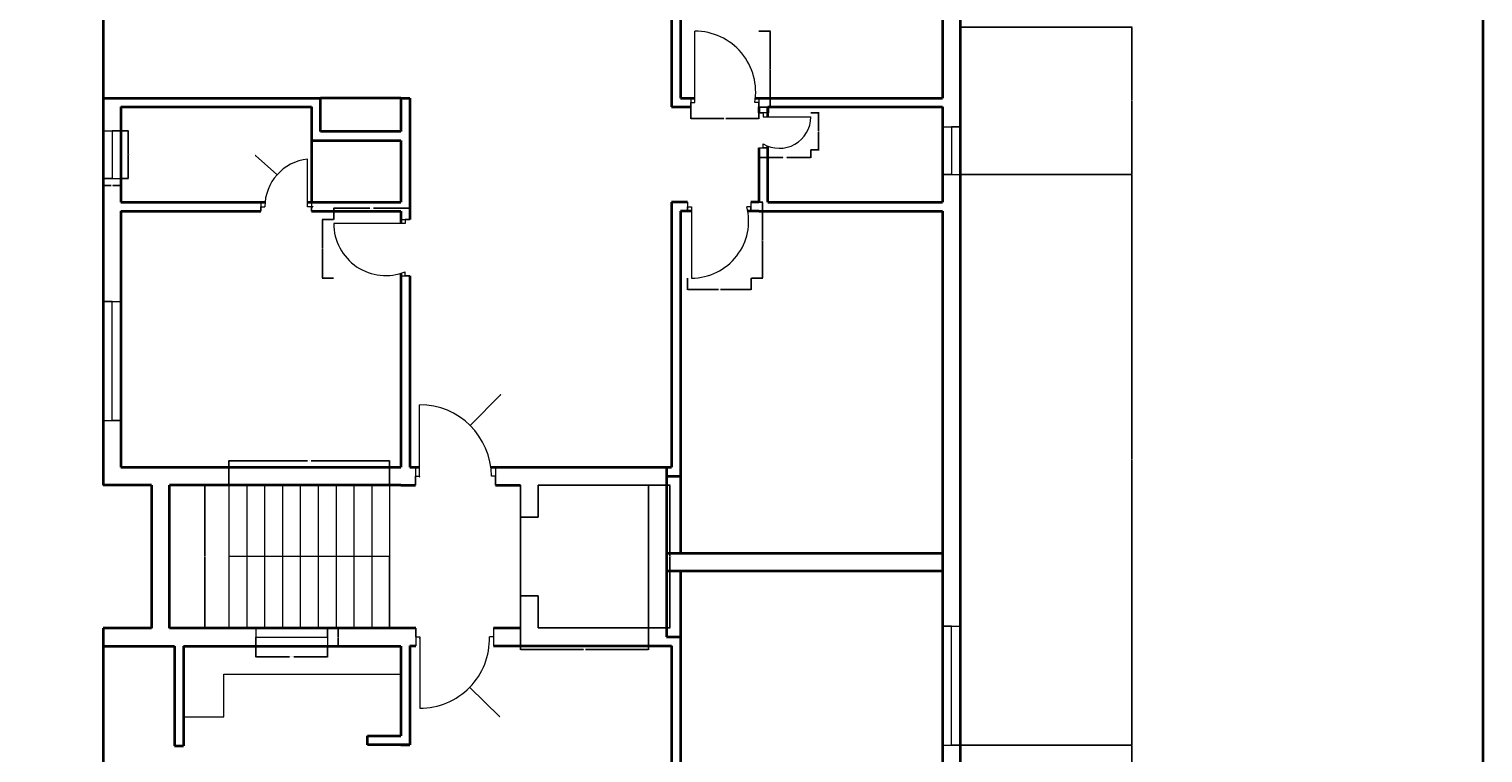
# Model space of a CAD drawing. Units: inches. Extents: x 2250 to 3547, y 1387 to 2604.
# Tile 5 of 11: x 2814 to 3547, y 1765 to 2129. Entities that reach past the tile are written whole.
import ezdxf

# ---------------------------------------------------------------- set-up
doc = ezdxf.new("R2010")
doc.units = ezdxf.units.IN
for name, color, linetype, lineweight in [('A-ANNO-DIMS', 2, 'Continuous', 18), ('A-ANNO-TTLB', 7, 'Continuous', 35), ('A-DOOR', 3, 'Continuous', 18), ('A-FLOR-CASE', 9, 'Continuous', 18), ('A-FLOR-EVTR', 6, 'Continuous', 25), ('A-FLOR-STRS', 7, 'Continuous', 18), ('A-GLAZ', 4, 'Continuous', 18), ('A-WALL', 7, 'Continuous', 35)]:
    doc.layers.add(name, color=color, linetype=linetype, lineweight=lineweight)
doc.styles.get("Standard").update_dxf_attribs({"font": 'arial.ttf'})
doc.dimstyles.get("Standard").update_dxf_attribs({"dimtxt": 0.18, "dimasz": 0.18, "dimexe": 0.18, "dimexo": 0.0625, "dimgap": 0.09, "dimtad": 0, "dimtih": 1, "dimtoh": 1, "dimdec": 4, "dimzin": 0, "dimdsep": 46, "dimtxsty": 'Standard', "dimcen": 0.09, "dimadec": 0, "dimazin": 0, "dimtfac": 1, "dimtdec": 4, "dimtofl": 0, "dimtmove": 0, "dimatfit": 3, "dimfxl": 1, "dimtolj": 1, "dimtzin": 0, "dimarcsym": 0})

# ---------------------------------------------------------------- blocks, each defined once
blk = doc.blocks.new('WIN-24')
for p, q in [((0, 24), (9, 24)), ((9, 24), (4.5, 24)), ((4.5, 24), (4.5, 0)), ((4.5, 0), (0, 0)), ((0, 0), (9, 0))]:
    blk.add_line(p, q)
blk = doc.blocks.new('WIN-60')
for p, q in [((0, 9), (0, 0)), ((60, 4.5), (60, 9)), ((60, 9), (60, 0)), ((0, 0), (0, 4.5)), ((0, 4.5), (60, 4.5))]:
    blk.add_line(p, q)
blk = doc.blocks.new('WIN-36')
for p, q in [((0, 9), (0, 0)), ((36, 4.5), (36, 9)), ((36, 9), (36, 0)), ((0, 0), (0, 4.5)), ((0, 4.5), (36, 4.5))]:
    blk.add_line(p, q)
blk = doc.blocks.new('DOOR-BED-NORTHEAST')
for p, q in [((2, 2.25), (2, 38.25)), ((0, 4.5), (0, 0)), ((0, 0), (0, 2.25)), ((0, 2.25), (2, 2.25)), ((34.25, 2.25), (32.25, 2.25)), ((34.25, 4.5), (34.25, 0)), ((34.25, 0), (34.25, 2.25))]:
    blk.add_line(p, q)
blk.add_arc((2, 7.54), 30.71, 350.07545, 90)
blk = doc.blocks.new('DOOR-BED-WEST-N')
for p, q in [((36, 26.33), (0, 26.33)), ((33.75, 28.33), (38.25, 28.33)), ((38.25, 28.33), (36, 28.33)), ((36, 28.33), (36, 26.33)), ((33.75, 0), (38.25, 0)), ((36, 0), (36, 2)), ((38.25, 0), (36, 0))]:
    blk.add_line(p, q)
blk.add_arc((26.22, 26.33), 26.22, 180, 291.89526)
blk = doc.blocks.new('DOOR-BATH-WEST-N')
for p, q in [((23.5, 2.25), (23.5, 26.25)), ((0, 4.5), (0, 0)), ((0, 0), (0, 2.25)), ((0, 2.25), (2, 2.25)), ((25.5, 2.25), (23.5, 2.25)), ((25.5, 4.5), (25.5, 0)), ((25.5, 0), (25.5, 2.25))]:
    blk.add_line(p, q)
blk.add_arc((26.15, 2.25), 24.15, 96.28991, 180)
blk = doc.blocks.new('DOOR-BATH-EAST-N')
for p, q in [((4.5, 17.63), (0, 17.63)), ((0, 17.63), (2.25, 17.63)), ((2.25, 17.63), (2.25, 15.63)), ((2.25, 15.63), (26.25, 15.63)), ((0, 0), (4.5, 0)), ((2.25, 0), (2.25, 2)), ((4.5, 0), (2.25, 0))]:
    blk.add_line(p, q)
blk.add_arc((10.38, 15.63), 15.87, 239.20063, 0)
blk = doc.blocks.new('DOOR-BED-EAST-N')
for p, q in [((0, 38.25), (0, 33.75)), ((31.84, 38.25), (31.84, 33.75)), ((0, 33.75), (0, 36)), ((0, 36), (2, 36)), ((2, 36), (2, 0)), ((31.84, 36), (29.84, 36)), ((31.84, 33.75), (31.84, 36))]:
    blk.add_line(p, q)
blk.add_arc((2, 28.77), 28.77, 270, 14.56312)
blk = doc.blocks.new('DOOR-LOBBY-NORTH')
for p, q in [((2, 4.5), (2, 40.5)), ((0, 9), (0, 0)), ((40.31, 9), (40.31, 0)), ((0, 0), (0, 4.5)), ((0, 4.5), (2, 4.5)), ((40.31, 4.5), (38.31, 4.5)), ((40.31, 0), (40.31, 4.5))]:
    blk.add_line(p, q)
blk.add_arc((2, 4.19), 36.31, 0.49224, 90)
blk = doc.blocks.new('DOOR-LOBBY-SOUTH')
for p, q in [((0, 36), (0, 40.36)), ((0, 40.36), (0, 31.5)), ((39.15, 40.5), (39.15, 31.5)), ((0, 36), (2, 36)), ((2, 36), (2, 0)), ((39.15, 36), (37.15, 36))]:
    blk.add_line(p, q)
blk.add_arc((2, 35.16), 35.16, 270, 1.37212)
blk = doc.blocks.new('STAIR-FLIGHT')
for p, q in [((0, 72.14), (0, 0)), ((9, 72.14), (9, 0)), ((18, 72.14), (18, 0)), ((27, 72.14), (27, 0)), ((36, 72.14), (36, 0)), ((45, 72.14), (45, 0)), ((54, 72.14), (54, 0)), ((63, 72.14), (63, 0)), ((72, 72.14), (72, 0)), ((81, 72.14), (81, 0)), ((81, 36.07), (0, 36.07)), ((81, 0), (81, 36.07))]:
    blk.add_line(p, q)
blk = doc.blocks.new('LIFT-SHAFT')
for p, q in [((0, 72), (0, 55.86)), ((9, 72), (60, 72)), ((9, 55.86), (9, 72)), ((60, 72), (64.53, 72)), ((64.53, 72), (64.53, 0)), ((0, 55.86), (9, 55.86)), ((0, 55.86), (0, 16.11)), ((0, 16.11), (9, 16.11)), ((0, 16.11), (0, 0)), ((9, 0), (9, 16.11)), ((60, 0), (9, 0)), ((9, 0), (60, 0)), ((64.53, 0), (60, 0))]:
    blk.add_line(p, q)
blk = doc.blocks.new('*D26')
at = {"layer": 'A-ANNO-DIMS', "color": 0, "lineweight": -2, "transparency": 16777216}
for p, q in [((2860.69, 2078.09), (2864.41, 2078.09)), ((2864.23, 2077.91), (2864.23, 2066.27)), ((2864.23, 2054.27), (2864.23, 2065.91)), ((2860.69, 2054.09), (2864.41, 2054.09))]:
    blk.add_line(p, q, dxfattribs=at)
at = {"layer": 'A-ANNO-DIMS', "color": 0, "transparency": 16777216}
for points in [[(2864.2, 2077.91), (2864.26, 2077.91), (2864.23, 2078.09)], [(2864.2, 2054.27), (2864.26, 2054.27), (2864.23, 2054.09)]]:
    blk.add_solid(points, dxfattribs=at)
at = {"layer": 'Defpoints', "color": 0, "transparency": 16777216}
for p in [(2860.63, 2078.09), (2864.23, 2078.09), (2860.63, 2054.09)]:
    blk.add_point(p, dxfattribs=at)
at = {"layer": 'A-ANNO-DIMS', "color": 0, "transparency": 16777216, "insert": (2864.23, 2066.09), "char_height": 0.18, "attachment_point": 5}
blk.add_mtext('\\A1;WINDOW 24 TYP.', dxfattribs=at)
blk = doc.blocks.new('*D27')
at = {"layer": 'A-ANNO-DIMS', "color": 0, "lineweight": -2, "transparency": 16777216}
for p, q in [((2851.63, 2054.03), (2851.63, 2050.31)), ((2860.63, 2054.03), (2860.63, 2050.31)), ((2851.81, 2050.49), (2855.67, 2050.49)), ((2860.45, 2050.49), (2856.59, 2050.49))]:
    blk.add_line(p, q, dxfattribs=at)
at = {"layer": 'A-ANNO-DIMS', "color": 0, "transparency": 16777216}
for points in [[(2851.81, 2050.52), (2851.81, 2050.46), (2851.63, 2050.49)], [(2860.45, 2050.52), (2860.45, 2050.46), (2860.63, 2050.49)]]:
    blk.add_solid(points, dxfattribs=at)
at = {"layer": 'Defpoints', "color": 0, "transparency": 16777216}
for p in [(2851.63, 2054.09), (2860.63, 2054.09), (2860.63, 2050.49)]:
    blk.add_point(p, dxfattribs=at)
at = {"layer": 'A-ANNO-DIMS', "color": 0, "transparency": 16777216, "insert": (2856.13, 2050.49), "char_height": 0.18, "attachment_point": 5}
blk.add_mtext('\\A1;9 TYP.', dxfattribs=at)
blk = doc.blocks.new('*D32')
at = {"layer": 'A-ANNO-DIMS', "color": 0, "lineweight": -2, "transparency": 16777216}
for p, q in [((2928.68, 1818.36), (2928.68, 1812.84)), ((2964.68, 1818.36), (2964.68, 1812.84)), ((2928.86, 1813.02), (2945.56, 1813.02)), ((2964.5, 1813.02), (2947.8, 1813.02))]:
    blk.add_line(p, q, dxfattribs=at)
at = {"layer": 'A-ANNO-DIMS', "color": 0, "transparency": 16777216}
for points in [[(2928.86, 1813.05), (2928.86, 1812.99), (2928.68, 1813.02)], [(2964.5, 1813.05), (2964.5, 1812.99), (2964.68, 1813.02)]]:
    blk.add_solid(points, dxfattribs=at)
at = {"layer": 'Defpoints', "color": 0, "transparency": 16777216}
for p in [(2928.68, 1818.42), (2964.68, 1818.42), (2964.68, 1813.02)]:
    blk.add_point(p, dxfattribs=at)
at = {"layer": 'A-ANNO-DIMS', "color": 0, "transparency": 16777216, "insert": (2946.68, 1813.02), "char_height": 0.18, "attachment_point": 5}
blk.add_mtext('\\A1;WINDOW 36 TYP.', dxfattribs=at)
blk = doc.blocks.new('*D33')
at = {"layer": 'A-ANNO-DIMS', "color": 0, "lineweight": -2, "transparency": 16777216}
for p, q in [((2964.74, 1827.42), (2970.26, 1827.42)), ((2970.08, 1827.24), (2970.08, 1823.11)), ((2964.74, 1818.42), (2970.26, 1818.42)), ((2970.08, 1818.6), (2970.08, 1822.74))]:
    blk.add_line(p, q, dxfattribs=at)
at = {"layer": 'A-ANNO-DIMS', "color": 0, "transparency": 16777216}
for points in [[(2970.05, 1827.24), (2970.11, 1827.24), (2970.08, 1827.42)], [(2970.05, 1818.6), (2970.11, 1818.6), (2970.08, 1818.42)]]:
    blk.add_solid(points, dxfattribs=at)
at = {"layer": 'Defpoints', "color": 0, "transparency": 16777216}
for p in [(2964.68, 1827.42), (2970.08, 1827.42), (2964.68, 1818.42)]:
    blk.add_point(p, dxfattribs=at)
at = {"layer": 'A-ANNO-DIMS', "color": 0, "transparency": 16777216, "insert": (2970.08, 1822.92), "char_height": 0.18, "attachment_point": 5}
blk.add_mtext('\\A1;9 TYP.', dxfattribs=at)
blk = doc.blocks.new('*D44')
at = {"layer": 'A-ANNO-DIMS', "color": 0, "lineweight": -2, "transparency": 16777216}
for p, q in [((3182.12, 2128.31), (3187.97, 2128.31)), ((3187.79, 2128.13), (3187.79, 2109.37)), ((3187.79, 2090.24), (3187.79, 2109.01)), ((3182.12, 2090.06), (3187.97, 2090.06))]:
    blk.add_line(p, q, dxfattribs=at)
at = {"layer": 'A-ANNO-DIMS', "color": 0, "transparency": 16777216}
for points in [[(3187.76, 2128.13), (3187.82, 2128.13), (3187.79, 2128.31)], [(3187.76, 2090.24), (3187.82, 2090.24), (3187.79, 2090.06)]]:
    blk.add_solid(points, dxfattribs=at)
at = {"layer": 'Defpoints', "color": 0, "transparency": 16777216}
for p in [(3182.05, 2128.31), (3187.79, 2128.31), (3182.05, 2090.06)]:
    blk.add_point(p, dxfattribs=at)
at = {"layer": 'A-ANNO-DIMS', "color": 0, "transparency": 16777216, "insert": (3187.79, 2109.19), "char_height": 0.18, "attachment_point": 5}
blk.add_mtext('\\A1;DOOR 38 TYP.', dxfattribs=at)
blk = doc.blocks.new('*D45')
at = {"layer": 'A-ANNO-DIMS', "color": 0, "lineweight": -2, "transparency": 16777216}
for p, q in [((3147.81, 2090), (3147.81, 2084.15)), ((3182.05, 2090), (3182.05, 2084.15)), ((3147.99, 2084.33), (3164.4, 2084.33)), ((3181.87, 2084.33), (3165.46, 2084.33))]:
    blk.add_line(p, q, dxfattribs=at)
at = {"layer": 'A-ANNO-DIMS', "color": 0, "transparency": 16777216}
for points in [[(3147.99, 2084.36), (3147.99, 2084.3), (3147.81, 2084.33)], [(3181.87, 2084.36), (3181.87, 2084.3), (3182.05, 2084.33)]]:
    blk.add_solid(points, dxfattribs=at)
at = {"layer": 'Defpoints', "color": 0, "transparency": 16777216}
for p in [(3147.81, 2090.06), (3182.05, 2090.06), (3182.05, 2084.33)]:
    blk.add_point(p, dxfattribs=at)
at = {"layer": 'A-ANNO-DIMS', "color": 0, "transparency": 16777216, "insert": (3164.93, 2084.33), "char_height": 0.18, "attachment_point": 5}
blk.add_mtext('\\A1;34 TYP.', dxfattribs=at)
blk = doc.blocks.new('*D48')
at = {"layer": 'A-ANNO-DIMS', "color": 0, "lineweight": -2, "transparency": 16777216}
for p, q in [((2967.88, 2033.38), (2967.88, 2039.24)), ((2968.06, 2039.06), (2986.07, 2039.06)), ((3005.95, 2039.06), (2987.94, 2039.06)), ((3006.13, 2033.38), (3006.13, 2039.24))]:
    blk.add_line(p, q, dxfattribs=at)
at = {"layer": 'A-ANNO-DIMS', "color": 0, "transparency": 16777216}
for points in [[(2968.06, 2039.09), (2968.06, 2039.03), (2967.88, 2039.06)], [(3005.95, 2039.09), (3005.95, 2039.03), (3006.13, 2039.06)]]:
    blk.add_solid(points, dxfattribs=at)
at = {"layer": 'Defpoints', "color": 0, "transparency": 16777216}
for p in [(3006.13, 2039.06), (2967.88, 2033.32), (3006.13, 2033.32)]:
    blk.add_point(p, dxfattribs=at)
at = {"layer": 'A-ANNO-DIMS', "color": 0, "transparency": 16777216, "insert": (2987, 2039.06), "char_height": 0.18, "attachment_point": 5}
blk.add_mtext('\\A1;DOOR 38 TYP.', dxfattribs=at)
blk = doc.blocks.new('*D49')
at = {"layer": 'A-ANNO-DIMS', "color": 0, "lineweight": -2, "transparency": 16777216}
for p, q in [((2967.82, 2033.32), (2961.96, 2033.32)), ((2962.14, 2033.14), (2962.14, 2018.71)), ((2962.14, 2003.92), (2962.14, 2018.35)), ((2967.82, 2003.74), (2961.96, 2003.74))]:
    blk.add_line(p, q, dxfattribs=at)
at = {"layer": 'A-ANNO-DIMS', "color": 0, "transparency": 16777216}
for points in [[(2962.11, 2033.14), (2962.17, 2033.14), (2962.14, 2033.32)], [(2962.11, 2003.92), (2962.17, 2003.92), (2962.14, 2003.74)]]:
    blk.add_solid(points, dxfattribs=at)
at = {"layer": 'Defpoints', "color": 0, "transparency": 16777216}
for p in [(2962.14, 2033.32), (2967.88, 2033.32), (2967.88, 2003.74)]:
    blk.add_point(p, dxfattribs=at)
at = {"layer": 'A-ANNO-DIMS', "color": 0, "transparency": 16777216, "insert": (2962.14, 2018.53), "char_height": 0.18, "attachment_point": 5}
blk.add_mtext('\\A1;30 TYP.', dxfattribs=at)
blk = doc.blocks.new('*D54')
at = {"layer": 'A-ANNO-DIMS', "color": 0, "lineweight": -2, "transparency": 16777216}
for p, q in [((3182.05, 2068.44), (3182.05, 2064.38)), ((3208.3, 2068.44), (3208.3, 2064.38)), ((3182.23, 2064.56), (3194.24, 2064.56)), ((3208.12, 2064.56), (3196.12, 2064.56))]:
    blk.add_line(p, q, dxfattribs=at)
at = {"layer": 'A-ANNO-DIMS', "color": 0, "transparency": 16777216}
for points in [[(3182.23, 2064.59), (3182.23, 2064.53), (3182.05, 2064.56)], [(3208.12, 2064.59), (3208.12, 2064.53), (3208.3, 2064.56)]]:
    blk.add_solid(points, dxfattribs=at)
at = {"layer": 'Defpoints', "color": 0, "transparency": 16777216}
for p in [(3182.05, 2068.5), (3208.3, 2068.5), (3208.3, 2064.56)]:
    blk.add_point(p, dxfattribs=at)
at = {"layer": 'A-ANNO-DIMS', "color": 0, "transparency": 16777216, "insert": (3195.18, 2064.56), "char_height": 0.18, "attachment_point": 5}
blk.add_mtext('\\A1;DOOR 26 TYP.', dxfattribs=at)
blk = doc.blocks.new('*D55')
at = {"layer": 'A-ANNO-DIMS', "color": 0, "lineweight": -2, "transparency": 16777216}
for p, q in [((3208.37, 2087.12), (3212.42, 2087.12)), ((3212.24, 2086.94), (3212.24, 2077.99)), ((3212.24, 2068.68), (3212.24, 2077.63)), ((3208.37, 2068.5), (3212.42, 2068.5))]:
    blk.add_line(p, q, dxfattribs=at)
at = {"layer": 'A-ANNO-DIMS', "color": 0, "transparency": 16777216}
for points in [[(3212.21, 2086.94), (3212.27, 2086.94), (3212.24, 2087.12)], [(3212.21, 2068.68), (3212.27, 2068.68), (3212.24, 2068.5)]]:
    blk.add_solid(points, dxfattribs=at)
at = {"layer": 'Defpoints', "color": 0, "transparency": 16777216}
for p in [(3208.3, 2087.12), (3212.24, 2087.12), (3208.3, 2068.5)]:
    blk.add_point(p, dxfattribs=at)
at = {"layer": 'A-ANNO-DIMS', "color": 0, "transparency": 16777216, "insert": (3212.24, 2077.81), "char_height": 0.18, "attachment_point": 5}
blk.add_mtext('\\A1;19 TYP.', dxfattribs=at)
blk = doc.blocks.new('*D56')
at = {"layer": 'A-ANNO-DIMS', "color": 0, "lineweight": -2, "transparency": 16777216}
for p, q in [((3178.32, 2042.06), (3184.18, 2042.06)), ((3184, 2041.88), (3184, 2023.12)), ((3184, 2003.99), (3184, 2022.76)), ((3178.32, 2003.81), (3184.18, 2003.81))]:
    blk.add_line(p, q, dxfattribs=at)
at = {"layer": 'A-ANNO-DIMS', "color": 0, "transparency": 16777216}
for points in [[(3183.97, 2041.88), (3184.03, 2041.88), (3184, 2042.06)], [(3183.97, 2003.99), (3184.03, 2003.99), (3184, 2003.81)]]:
    blk.add_solid(points, dxfattribs=at)
at = {"layer": 'Defpoints', "color": 0, "transparency": 16777216}
for p in [(3178.26, 2042.06), (3184, 2042.06), (3178.26, 2003.81)]:
    blk.add_point(p, dxfattribs=at)
at = {"layer": 'A-ANNO-DIMS', "color": 0, "transparency": 16777216, "insert": (3184, 2022.94), "char_height": 0.18, "attachment_point": 5}
blk.add_mtext('\\A1;DOOR 38 TYP.', dxfattribs=at)
blk = doc.blocks.new('*D57')
at = {"layer": 'A-ANNO-DIMS', "color": 0, "lineweight": -2, "transparency": 16777216}
for p, q in [((3146.18, 2003.75), (3146.18, 1997.9)), ((3178.26, 2003.75), (3178.26, 1997.9)), ((3146.36, 1998.08), (3161.69, 1998.08)), ((3178.08, 1998.08), (3162.75, 1998.08))]:
    blk.add_line(p, q, dxfattribs=at)
at = {"layer": 'A-ANNO-DIMS', "color": 0, "transparency": 16777216}
for points in [[(3146.36, 1998.11), (3146.36, 1998.05), (3146.18, 1998.08)], [(3178.08, 1998.11), (3178.08, 1998.05), (3178.26, 1998.08)]]:
    blk.add_solid(points, dxfattribs=at)
at = {"layer": 'Defpoints', "color": 0, "transparency": 16777216}
for p in [(3146.18, 2003.81), (3178.26, 2003.81), (3178.26, 1998.08)]:
    blk.add_point(p, dxfattribs=at)
at = {"layer": 'A-ANNO-DIMS', "color": 0, "transparency": 16777216, "insert": (3162.22, 1998.08), "char_height": 0.18, "attachment_point": 5}
blk.add_mtext('\\A1;32 TYP.', dxfattribs=at)
blk = doc.blocks.new('*D70')
at = {"layer": 'A-ANNO-DIMS', "color": 0, "lineweight": -2, "transparency": 16777216}
for p, q in [((2915.01, 1899.63), (2915.01, 1911.89)), ((2915.19, 1911.71), (2954.57, 1911.71)), ((2995.83, 1911.71), (2956.44, 1911.71)), ((2996.01, 1899.63), (2996.01, 1911.89))]:
    blk.add_line(p, q, dxfattribs=at)
at = {"layer": 'A-ANNO-DIMS', "color": 0, "transparency": 16777216}
for points in [[(2915.19, 1911.74), (2915.19, 1911.68), (2915.01, 1911.71)], [(2995.83, 1911.74), (2995.83, 1911.68), (2996.01, 1911.71)]]:
    blk.add_solid(points, dxfattribs=at)
at = {"layer": 'Defpoints', "color": 0, "transparency": 16777216}
for p in [(2996.01, 1911.71), (2915.01, 1899.56), (2996.01, 1899.56)]:
    blk.add_point(p, dxfattribs=at)
at = {"layer": 'A-ANNO-DIMS', "color": 0, "transparency": 16777216, "insert": (2955.51, 1911.71), "char_height": 0.18, "attachment_point": 5}
blk.add_mtext('\\A1;STAIR 81 TYP.', dxfattribs=at)
blk = doc.blocks.new('*D71')
at = {"layer": 'A-ANNO-DIMS', "color": 0, "lineweight": -2, "transparency": 16777216}
for p, q in [((2914.94, 1899.56), (2902.68, 1899.56)), ((2902.86, 1899.38), (2902.86, 1863.67)), ((2902.86, 1827.6), (2902.86, 1863.31)), ((2914.94, 1827.42), (2902.68, 1827.42))]:
    blk.add_line(p, q, dxfattribs=at)
at = {"layer": 'A-ANNO-DIMS', "color": 0, "transparency": 16777216}
for points in [[(2902.83, 1899.38), (2902.89, 1899.38), (2902.86, 1899.56)], [(2902.83, 1827.6), (2902.89, 1827.6), (2902.86, 1827.42)]]:
    blk.add_solid(points, dxfattribs=at)
at = {"layer": 'Defpoints', "color": 0, "transparency": 16777216}
for p in [(2902.86, 1899.56), (2915.01, 1899.56), (2915.01, 1827.42)]:
    blk.add_point(p, dxfattribs=at)
at = {"layer": 'A-ANNO-DIMS', "color": 0, "transparency": 16777216, "insert": (2902.86, 1863.49), "char_height": 0.18, "attachment_point": 5}
blk.add_mtext('\\A1;72 TYP.', dxfattribs=at)
blk = doc.blocks.new('*D72')
at = {"layer": 'A-ANNO-DIMS', "color": 0, "lineweight": -2, "transparency": 16777216}
for p, q in [((3126.55, 1899.56), (3137.47, 1899.56)), ((3137.29, 1899.38), (3137.29, 1863.75)), ((3137.29, 1827.74), (3137.29, 1863.38)), ((3126.55, 1827.56), (3137.47, 1827.56))]:
    blk.add_line(p, q, dxfattribs=at)
at = {"layer": 'A-ANNO-DIMS', "color": 0, "transparency": 16777216}
for points in [[(3137.26, 1899.38), (3137.32, 1899.38), (3137.29, 1899.56)], [(3137.26, 1827.74), (3137.32, 1827.74), (3137.29, 1827.56)]]:
    blk.add_solid(points, dxfattribs=at)
at = {"layer": 'Defpoints', "color": 0, "transparency": 16777216}
for p in [(3126.49, 1899.56), (3137.29, 1899.56), (3126.49, 1827.56)]:
    blk.add_point(p, dxfattribs=at)
at = {"layer": 'A-ANNO-DIMS', "color": 0, "transparency": 16777216, "insert": (3137.29, 1863.56), "char_height": 0.18, "attachment_point": 5}
blk.add_mtext('\\A1;LIFT SHAFT 72 TYP.', dxfattribs=at)
blk = doc.blocks.new('*D73')
at = {"layer": 'A-ANNO-DIMS', "color": 0, "lineweight": -2, "transparency": 16777216}
for p, q in [((3061.96, 1827.5), (3061.96, 1816.58)), ((3126.49, 1827.5), (3126.49, 1816.58)), ((3062.14, 1816.76), (3093.69, 1816.76)), ((3126.31, 1816.76), (3094.75, 1816.76))]:
    blk.add_line(p, q, dxfattribs=at)
at = {"layer": 'A-ANNO-DIMS', "color": 0, "transparency": 16777216}
for points in [[(3062.14, 1816.79), (3062.14, 1816.73), (3061.96, 1816.76)], [(3126.31, 1816.79), (3126.31, 1816.73), (3126.49, 1816.76)]]:
    blk.add_solid(points, dxfattribs=at)
at = {"layer": 'Defpoints', "color": 0, "transparency": 16777216}
for p in [(3061.96, 1827.56), (3126.49, 1827.56), (3126.49, 1816.76)]:
    blk.add_point(p, dxfattribs=at)
at = {"layer": 'A-ANNO-DIMS', "color": 0, "transparency": 16777216, "insert": (3094.22, 1816.76), "char_height": 0.18, "attachment_point": 5}
blk.add_mtext('\\A1;65 TYP.', dxfattribs=at)
blk = doc.blocks.new('*D85')
at = {"layer": 'A-ANNO-DIMS', "color": 0, "lineweight": -2, "transparency": 16777216}
for p, q in [((3001.57, 2245.18), (2779.34, 2245.18)), ((2779.52, 2245), (2779.52, 1894.73)), ((2779.52, 1544.1), (2779.52, 1894.37)), ((2851.57, 1543.92), (2779.34, 1543.92))]:
    blk.add_line(p, q, dxfattribs=at)
at = {"layer": 'A-ANNO-DIMS', "color": 0, "transparency": 16777216}
for points in [[(2779.49, 2245), (2779.55, 2245), (2779.52, 2245.18)], [(2779.49, 1544.1), (2779.55, 1544.1), (2779.52, 1543.92)]]:
    blk.add_solid(points, dxfattribs=at)
at = {"layer": 'Defpoints', "color": 0, "transparency": 16777216}
for p in [(2779.52, 2245.18), (3001.63, 2245.18), (2851.63, 1543.92)]:
    blk.add_point(p, dxfattribs=at)
at = {"layer": 'A-ANNO-DIMS', "color": 0, "transparency": 16777216, "insert": (2779.52, 1894.55), "char_height": 0.18, "attachment_point": 5}
blk.add_mtext('\\A1;701.3', dxfattribs=at)
blk = doc.blocks.new('*D88')
at = {"layer": 'A-ANNO-DIMS', "color": 0, "lineweight": -2, "transparency": 16777216}
for p, q in [((3283.69, 1768.42), (3370.22, 1768.42)), ((3370.04, 1768.24), (3370.04, 1728.59)), ((3370.04, 1688.57), (3370.04, 1728.23)), ((3283.69, 1688.39), (3370.22, 1688.39))]:
    blk.add_line(p, q, dxfattribs=at)
at = {"layer": 'A-ANNO-DIMS', "color": 0, "transparency": 16777216}
for points in [[(3370.01, 1768.24), (3370.07, 1768.24), (3370.04, 1768.42)], [(3370.01, 1688.57), (3370.07, 1688.57), (3370.04, 1688.39)]]:
    blk.add_solid(points, dxfattribs=at)
at = {"layer": 'Defpoints', "color": 0, "transparency": 16777216}
for p in [(3283.63, 1768.42), (3370.04, 1768.42), (3283.63, 1688.39)]:
    blk.add_point(p, dxfattribs=at)
at = {"layer": 'A-ANNO-DIMS', "color": 0, "transparency": 16777216, "insert": (3370.04, 1728.41), "char_height": 0.18, "attachment_point": 5}
blk.add_mtext('\\A1;80.03', dxfattribs=at)
blk = doc.blocks.new('*D89')
at = {"layer": 'A-ANNO-DIMS', "color": 0, "lineweight": -2, "transparency": 16777216}
for p, q in [((3283.69, 2056.05), (3370.22, 2056.05)), ((3370.04, 2055.87), (3370.04, 1912.42)), ((3370.04, 1768.6), (3370.04, 1912.06)), ((3283.69, 1768.42), (3370.22, 1768.42))]:
    blk.add_line(p, q, dxfattribs=at)
at = {"layer": 'A-ANNO-DIMS', "color": 0, "transparency": 16777216}
for points in [[(3370.01, 2055.87), (3370.07, 2055.87), (3370.04, 2056.05)], [(3370.01, 1768.6), (3370.07, 1768.6), (3370.04, 1768.42)]]:
    blk.add_solid(points, dxfattribs=at)
at = {"layer": 'Defpoints', "color": 0, "transparency": 16777216}
for p in [(3283.63, 2056.05), (3370.04, 2056.05), (3283.63, 1768.42)]:
    blk.add_point(p, dxfattribs=at)
at = {"layer": 'A-ANNO-DIMS', "color": 0, "transparency": 16777216, "insert": (3370.04, 1912.24), "char_height": 0.18, "attachment_point": 5}
blk.add_mtext('\\A1;287.6', dxfattribs=at)
blk = doc.blocks.new('*D90')
at = {"layer": 'A-ANNO-DIMS', "color": 0, "lineweight": -2, "transparency": 16777216}
for p, q in [((3283.69, 2130.34), (3370.22, 2130.34)), ((3370.04, 2130.16), (3370.04, 2093.38)), ((3370.04, 2056.23), (3370.04, 2093.01)), ((3283.69, 2056.05), (3370.22, 2056.05))]:
    blk.add_line(p, q, dxfattribs=at)
at = {"layer": 'A-ANNO-DIMS', "color": 0, "transparency": 16777216}
for points in [[(3370.01, 2130.16), (3370.07, 2130.16), (3370.04, 2130.34)], [(3370.01, 2056.23), (3370.07, 2056.23), (3370.04, 2056.05)]]:
    blk.add_solid(points, dxfattribs=at)
at = {"layer": 'Defpoints', "color": 0, "transparency": 16777216}
for p in [(3283.63, 2130.34), (3370.04, 2130.34), (3283.63, 2056.05)]:
    blk.add_point(p, dxfattribs=at)
at = {"layer": 'A-ANNO-DIMS', "color": 0, "transparency": 16777216, "insert": (3370.04, 2093.2), "char_height": 0.18, "attachment_point": 5}
blk.add_mtext('\\A1;74.29', dxfattribs=at)
blk = doc.blocks.new('*D114')
at = {"layer": 'A-ANNO-DIMS', "color": 0, "lineweight": -2, "transparency": 16777216}
for p, q in [((3051.96, 1945.01), (3036.75, 1929.67)), ((3052.14, 1945.01), (3051.96, 1945.01)), ((3010.96, 1903.75), (3011.14, 1903.75)), ((3011.05, 1903.66), (3011.05, 1903.84))]:
    blk.add_line(p, q, dxfattribs=at)
at = {"layer": 'A-ANNO-DIMS', "color": 0, "transparency": 16777216}
blk.add_solid([(3036.73, 1929.69), (3036.77, 1929.64), (3036.62, 1929.54)], dxfattribs=at)
at = {"layer": 'Defpoints', "color": 0, "transparency": 16777216}
for p in [(3036.62, 1929.54), (3011.05, 1903.75)]:
    blk.add_point(p, dxfattribs=at)
at = {"layer": 'A-ANNO-DIMS', "color": 0, "transparency": 16777216, "insert": (3052.6, 1945.01), "char_height": 0.18, "attachment_point": 5}
blk.add_mtext('\\A1;R36.31', dxfattribs=at)
blk = doc.blocks.new('*D115')
at = {"layer": 'A-ANNO-DIMS', "color": 0, "lineweight": -2, "transparency": 16777216}
for p, q in [((3011.12, 1822.22), (3011.3, 1822.22)), ((3011.21, 1822.13), (3011.21, 1822.31)), ((3051.46, 1782.92), (3036.5, 1797.54)), ((3051.64, 1782.92), (3051.46, 1782.92))]:
    blk.add_line(p, q, dxfattribs=at)
at = {"layer": 'A-ANNO-DIMS', "color": 0, "transparency": 16777216}
blk.add_solid([(3036.52, 1797.56), (3036.48, 1797.51), (3036.37, 1797.66)], dxfattribs=at)
at = {"layer": 'Defpoints', "color": 0, "transparency": 16777216}
for p in [(3011.21, 1822.22), (3036.37, 1797.66)]:
    blk.add_point(p, dxfattribs=at)
at = {"layer": 'A-ANNO-DIMS', "color": 0, "transparency": 16777216, "insert": (3052.12, 1782.92), "char_height": 0.18, "attachment_point": 5}
blk.add_mtext('\\A1;R35.16', dxfattribs=at)
blk = doc.blocks.new('*D126')
at = {"layer": 'A-ANNO-DIMS', "color": 0, "lineweight": -2, "transparency": 16777216}
for p, q in [((2928.32, 2065.59), (2928.5, 2065.59)), ((2928.5, 2065.59), (2939.16, 2056.05)), ((2957.18, 2039.81), (2957.36, 2039.81)), ((2957.27, 2039.72), (2957.27, 2039.9))]:
    blk.add_line(p, q, dxfattribs=at)
at = {"layer": 'A-ANNO-DIMS', "color": 0, "transparency": 16777216}
blk.add_solid([(2939.18, 2056.07), (2939.14, 2056.02), (2939.29, 2055.93)], dxfattribs=at)
at = {"layer": 'Defpoints', "color": 0, "transparency": 16777216}
for p in [(2939.29, 2055.93), (2957.27, 2039.81)]:
    blk.add_point(p, dxfattribs=at)
at = {"layer": 'A-ANNO-DIMS', "color": 0, "transparency": 16777216, "insert": (2927.77, 2065.59), "char_height": 0.18, "attachment_point": 5}
blk.add_mtext('\\A1;R24.145', dxfattribs=at)

msp = doc.modelspace()

# ---------------------------------------------------------------- linework, layer by layer
at = {"layer": 'A-ANNO-TTLB'}
msp.add_lwpolyline([(2250.1093, 2604.1988), (3546.995, 2604.1988), (3546.995, 1386.7251), (2250.1093, 1386.7251)], close=True, dxfattribs=at)
at = {"layer": 'A-FLOR-CASE'}
for p, q in [((2912.5208, 1782.7382), (2912.5208, 1804.325)), ((2912.5208, 1804.325), (3001.6288, 1804.325)), ((2892.1288, 1782.7382), (2912.5208, 1782.7382))]:
    msp.add_line(p, q, dxfattribs=at)
at = {"layer": 'A-WALL'}
for p, q in [((2851.6288, 2232.5639), (2851.6288, 1899.5639)), ((2851.6288, 2232.5639), (2851.6288, 1899.5639)), ((3283.6288, 2232.5639), (3283.6288, 1543.9245)), ((3142.6288, 2223.5639), (3142.6288, 2094.5639)), ((3274.6288, 2223.5639), (3274.6288, 2094.5639)), ((3138.1288, 2198.6762), (3138.1288, 2090.0639)), ((2851.6288, 2094.5639), (2961.1288, 2094.5639)), ((2860.6288, 2090.0639), (2860.6288, 2042.0639)), ((2860.6288, 2090.0639), (2956.6288, 2090.0639)), ((2860.6288, 2090.0639), (2956.6288, 2090.0639)), ((2956.6288, 2090.0639), (2956.6288, 2042.0639)), ((2961.1288, 2077.6358), (2961.1288, 2094.5639)), ((3001.6288, 2094.5639), (2961.1288, 2094.5639)), ((3001.6288, 2094.5639), (3001.6288, 2077.6358)), ((3001.6288, 2094.5639), (3006.1288, 2094.5639)), ((3006.1288, 2094.5639), (3006.1288, 2033.3217)), ((3138.1288, 2090.0639), (3147.8068, 2090.0639)), ((3142.6288, 2094.5639), (3149.8068, 2094.5639)), ((3180.3632, 2094.5639), (3274.6288, 2094.5639)), ((3182.0548, 2090.0639), (3182.0548, 2087.1197)), ((3186.5548, 2090.0639), (3274.6288, 2090.0639)), ((3186.5548, 2085.1197), (3186.5548, 2090.0639)), ((3186.5548, 2090.0639), (3186.5548, 2087.1197)), ((3274.6288, 2090.0639), (3274.6288, 2042.0639)), ((3001.6288, 2077.6358), (2961.1288, 2077.6358)), ((2956.6288, 2073.1358), (3001.6288, 2073.1358)), ((3001.6288, 2073.1358), (3001.6288, 2042.0639)), ((3182.0548, 2069.4856), (3182.0548, 2042.0639)), ((3186.5548, 2042.0639), (3186.5548, 2070.3753)), ((2860.6288, 2042.0639), (2933.2338, 2042.0639)), ((2860.6288, 2037.5639), (2860.6288, 1908.5639)), ((2860.6288, 2037.5639), (2931.1288, 2037.5639)), ((2860.6288, 2037.5639), (2860.6288, 1908.5639)), ((2954.6288, 2042.0639), (3001.6288, 2042.0639)), ((2956.6288, 2037.5639), (3001.6288, 2037.5639)), ((3001.6288, 2037.5639), (3001.6288, 2031.3217)), ((3138.1288, 2042.0639), (3138.1288, 1908.5639)), ((3146.1776, 2042.0639), (3138.1288, 2042.0639)), ((3142.6288, 2037.5639), (3142.6288, 1908.5639)), ((3148.1776, 2037.5639), (3142.6288, 2037.5639)), ((3182.0548, 2037.5639), (3176.5094, 2037.5639)), ((3182.0548, 2042.0639), (3178.0201, 2042.0639)), ((3182.0548, 2037.5639), (3274.6288, 2037.5639)), ((3182.0548, 2037.5639), (3186.5548, 2037.5639)), ((3186.5548, 2042.0639), (3274.6288, 2042.0639)), ((3274.6288, 2037.5639), (3274.6288, 1727.1967)), ((3001.6288, 2006.204), (3001.6288, 1908.5639)), ((3006.1288, 2004.9915), (3006.1288, 1908.5639)), ((2860.6288, 1908.5639), (3001.6288, 1908.5639)), ((3006.1288, 1908.5639), (3011.0537, 1908.5639)), ((3047.0454, 1908.5639), (3138.1288, 1908.5639)), ((3126.4871, 1908.5639), (3135.4871, 1908.5639)), ((3135.4871, 1908.5639), (3135.4871, 1823.0639)), ((3135.4871, 1908.5639), (3135.4871, 1904.0639)), ((3142.6288, 1908.5639), (3142.6288, 1865.1967)), ((2876.0158, 1899.5639), (2851.6288, 1899.5639)), ((2876.0158, 1899.5639), (2876.0158, 1827.4245)), ((3001.6288, 1899.5639), (2885.0158, 1899.5639)), ((2885.0158, 1827.4245), (2885.0158, 1899.5639)), ((3001.6288, 1899.5639), (3006.1288, 1899.5639)), ((3006.1288, 1899.5639), (3009.0537, 1899.5639)), ((3049.3643, 1899.5639), (3061.9563, 1899.5639)), ((3135.4871, 1904.0639), (3142.6288, 1904.0639)), ((3135.4871, 1865.1967), (3274.6288, 1865.1967)), ((3274.6288, 1865.1967), (3274.6288, 1856.1967)), ((3274.6288, 1856.1967), (3135.4871, 1856.1967)), ((3142.6288, 1856.1967), (3142.6288, 1727.1967)), ((2851.6288, 1827.4245), (2851.6288, 1543.9245)), ((2851.6288, 1827.4245), (2851.6288, 1543.9245)), ((2876.0158, 1827.4245), (2851.6288, 1827.4245)), ((2851.6288, 1827.4245), (2851.6288, 1818.4245)), ((3009.2144, 1827.4245), (2885.0158, 1827.4245)), ((3048.3624, 1827.5639), (3061.9563, 1827.5639)), ((2851.6288, 1818.4245), (2887.6288, 1818.4245)), ((2887.6288, 1818.4245), (2887.6288, 1768.2118)), ((2892.1288, 1818.4245), (2892.1288, 1768.2118)), ((2892.1288, 1818.4245), (3001.6288, 1818.4245)), ((3001.6288, 1818.4245), (3001.6288, 1773.2235)), ((3006.1288, 1818.5639), (3006.1288, 1768.7235)), ((3006.1288, 1818.5639), (3009.2144, 1818.5639)), ((3048.3624, 1818.5639), (3138.1288, 1818.5639)), ((3135.4871, 1823.0639), (3142.6288, 1823.0639)), ((3138.1288, 1818.5639), (3138.1288, 1722.6967)), ((2984.9084, 1768.7235), (2984.9084, 1773.2235)), ((2984.9084, 1773.2235), (3001.6288, 1773.2235)), ((2887.6288, 1768.2118), (2892.1288, 1768.2118)), ((3006.1288, 1768.7235), (2984.9084, 1768.7235)), ((3001.6288, 1768.7235), (3006.1288, 1768.7235))]:
    msp.add_line(p, q, dxfattribs=at)

# ---------------------------------------------------------------- block references
at = {"layer": 'A-DOOR'}
for name, p in [('DOOR-BED-NORTHEAST', (3147.8068, 2090.0639)), ('DOOR-BATH-EAST-N', (3182.0548, 2069.4856)), ('DOOR-BATH-WEST-N', (2931.1288, 2037.5639)), ('DOOR-BED-EAST-N', (3146.1776, 2003.8139)), ('DOOR-BED-WEST-N', (2967.8788, 2004.9915)), ('DOOR-LOBBY-NORTH', (3009.0537, 1899.5639)), ('DOOR-LOBBY-SOUTH', (3009.2144, 1787.0639))]:
    msp.add_blockref(name, p, dxfattribs=at)
at = {"layer": 'A-FLOR-EVTR'}
msp.add_blockref('LIFT-SHAFT', (3061.9563, 1827.5639), dxfattribs=at)
at = {"layer": 'A-FLOR-STRS'}
msp.add_blockref('STAIR-FLIGHT', (2915.0059, 1827.4245), dxfattribs=at)
at = {"layer": 'A-GLAZ'}
for name, p in [('WIN-24', (2851.6288, 2054.091)), ('WIN-24', (3274.6288, 2056.0503)), ('WIN-36', (2928.6807, 1818.4245))]:
    msp.add_blockref(name, p, dxfattribs=at)
for p, rotation in [((2860.6288, 1932.0574), 90.00000000000072), ((3283.6288, 1768.424), 90.00000000000146)]:
    msp.add_blockref('WIN-60', p, dxfattribs=dict(at, rotation=rotation))

# ---------------------------------------------------------------- dimensions: what is measured, and where the dimension line sits
at = {"layer": 'A-ANNO-DIMS'}
for base, p1, p2, override, picture, middle in [((2779.5165, 2245.1762), (2851.6288, 1543.9245), (3001.6288, 2245.1762), {"dimdec": 1, "dimlfac": 1, "dimrnd": 0, "dimzin": 0, "dimdsep": 46, "dimlunit": 2}, '*D85', (2779.5165, 1894.5504)), ((3370.0441, 2130.3411), (3283.6288, 2056.0503), (3283.6288, 2130.3411), {"dimdec": 2, "dimlfac": 1, "dimrnd": 0, "dimzin": 0, "dimdsep": 46, "dimlunit": 2}, '*D90', (3370.0441, 2093.1957)), ((3370.0441, 2056.0503), (3283.6288, 1768.424), (3283.6288, 2056.0503), {"dimdec": 1, "dimlfac": 1, "dimrnd": 0, "dimzin": 0, "dimdsep": 46, "dimlunit": 2}, '*D89', (3370.0441, 1912.2372)), ((3370.0441, 1768.424), (3283.6288, 1688.3924), (3283.6288, 1768.424), {"dimdec": 2, "dimlfac": 1, "dimrnd": 0, "dimzin": 0, "dimdsep": 46, "dimlunit": 2}, '*D88', (3370.0441, 1728.4082))]:
    dim = msp.add_linear_dim(base=base, p1=p1, p2=p2, angle=90, dimstyle='Standard', override=override, dxfattribs=at)
    dim.commit()
    dim.dimension.update_dxf_attribs({"geometry": picture, "text_midpoint": middle})
for base, p1, p2, text, picture, middle in [((3187.7923, 2128.3139), (3182.0548, 2090.0639), (3182.0548, 2128.3139), 'DOOR <> TYP.', '*D44', (3187.7923, 2109.1889)), ((3212.2423, 2087.1197), (3208.3048, 2068.4979), (3208.3048, 2087.1197), '<> TYP.', '*D55', (3212.2423, 2077.8088)), ((2864.2288, 2078.091), (2860.6288, 2054.091), (2860.6288, 2078.091), 'WINDOW <> TYP.', '*D26', (2864.2288, 2066.091)), ((3183.9967, 2042.0639), (3178.2592, 2003.8139), (3178.2592, 2042.0639), 'DOOR <> TYP.', '*D56', (3183.9967, 2022.9389)), ((2962.1413, 2033.3217), (2967.8788, 2003.744), (2967.8788, 2033.3217), '<> TYP.', '*D49', (2962.1413, 2018.5328)), ((2902.8559, 1899.5639), (2915.0059, 1827.4245), (2915.0059, 1899.5639), '<> TYP.', '*D71', (2902.8559, 1863.4942)), ((3137.2871, 1899.5639), (3126.4871, 1827.5639), (3126.4871, 1899.5639), 'LIFT SHAFT <> TYP.', '*D72', (3137.2871, 1863.5639)), ((2970.0807, 1827.4245), (2964.6807, 1818.4245), (2964.6807, 1827.4245), '<> TYP.', '*D33', (2970.0807, 1822.9245))]:
    dim = msp.add_linear_dim(base=base, p1=p1, p2=p2, angle=90, text=text, dimstyle='Standard', override={"dimdec": 0, "dimlfac": 1, "dimrnd": 0, "dimzin": 0, "dimdsep": 46, "dimlunit": 2}, dxfattribs=at)
    dim.commit()
    dim.dimension.update_dxf_attribs({"geometry": picture, "text_midpoint": middle})
for base, p1, p2, text, picture, middle in [((3182.0548, 2084.3264), (3147.8068, 2090.0639), (3182.0548, 2090.0639), '<> TYP.', '*D45', (3164.9308, 2084.3264)), ((3208.3048, 2064.5604), (3182.0548, 2068.4979), (3208.3048, 2068.4979), 'DOOR <> TYP.', '*D54', (3195.1798, 2064.5604)), ((2860.6288, 2050.491), (2851.6288, 2054.091), (2860.6288, 2054.091), '<> TYP.', '*D27', (2856.1288, 2050.491)), ((3006.1288, 2039.0592), (2967.8788, 2033.3217), (3006.1288, 2033.3217), 'DOOR <> TYP.', '*D48', (2987.0038, 2039.0592)), ((3178.2592, 1998.0764), (3146.1776, 2003.8139), (3178.2592, 2003.8139), '<> TYP.', '*D57', (3162.2184, 1998.0764)), ((2996.0059, 1911.7139), (2915.0059, 1899.5639), (2996.0059, 1899.5639), 'STAIR <> TYP.', '*D70', (2955.5059, 1911.7139)), ((3126.4871, 1816.7639), (3061.9563, 1827.5639), (3126.4871, 1827.5639), '<> TYP.', '*D73', (3094.2217, 1816.7639)), ((2964.6807, 1813.0245), (2928.6807, 1818.4245), (2964.6807, 1818.4245), 'WINDOW <> TYP.', '*D32', (2946.6807, 1813.0245))]:
    dim = msp.add_linear_dim(base=base, p1=p1, p2=p2, text=text, dimstyle='Standard', override={"dimdec": 0, "dimlfac": 1, "dimrnd": 0, "dimzin": 0, "dimdsep": 46, "dimlunit": 2}, dxfattribs=at)
    dim.commit()
    dim.dimension.update_dxf_attribs({"geometry": picture, "text_midpoint": middle})
for center, mpoint, override, picture, middle in [((2957.2741, 2039.8139), (2939.29, 2055.925), {"dimdec": 3, "dimlfac": 1, "dimrnd": 0, "dimzin": 0, "dimdsep": 46, "dimlunit": 2}, '*D126', (2927.769, 2065.5917)), ((3011.0537, 1903.752), (3036.62, 1929.538), {"dimdec": 2, "dimlfac": 1, "dimrnd": 0, "dimzin": 0, "dimdsep": 46, "dimlunit": 2}, '*D114', (3052.6023, 1945.0097)), ((3011.2144, 1822.222), (3036.3709, 1797.6611), {"dimdec": 2, "dimlfac": 1, "dimrnd": 0, "dimzin": 0, "dimdsep": 46, "dimlunit": 2}, '*D115', (3052.1246, 1782.9245))]:
    dim = msp.add_radius_dim(center=center, mpoint=mpoint, dimstyle='Standard', override=override, dxfattribs=at)
    dim.commit()
    dim.dimension.update_dxf_attribs({"geometry": picture, "text_midpoint": middle, "dimtype": 164})

doc.saveas('drawing.dxf')
